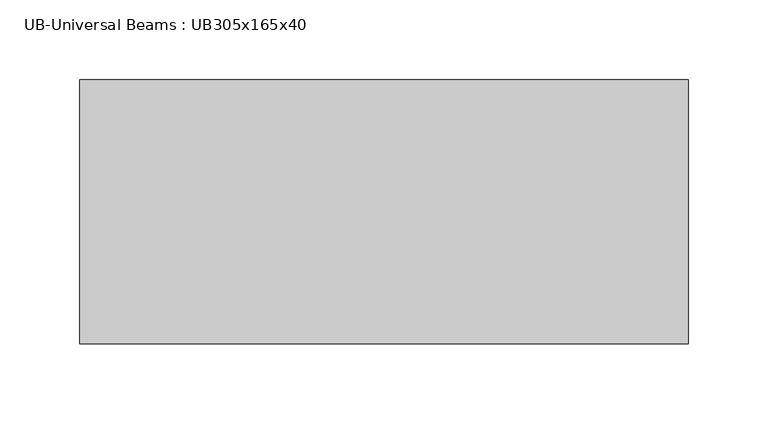
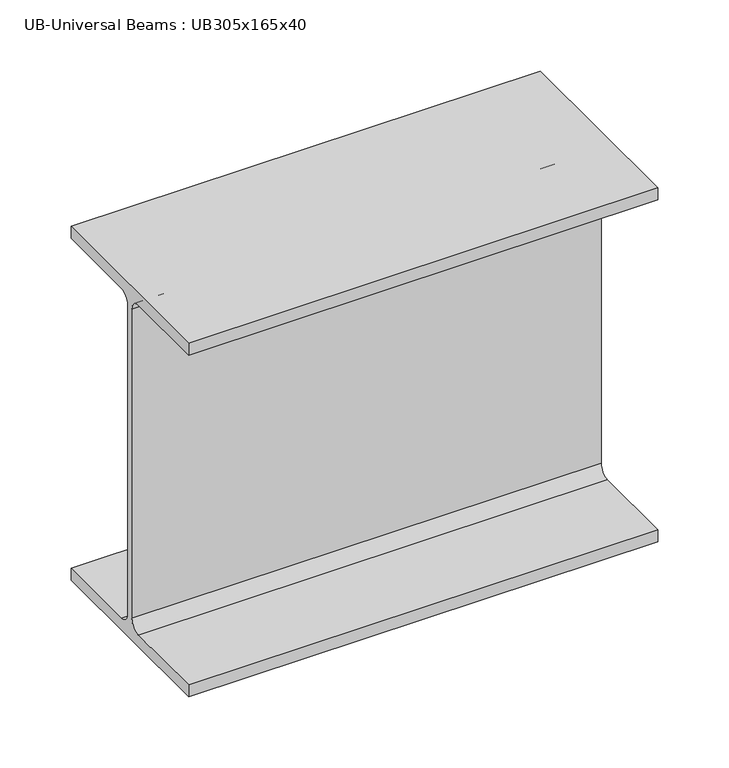
"""IFC4 building model written with IfcOpenShell, lengths in millimetres: beam geometry, UB-Universal Beams : UB305x165x40."""

from ifc_helpers import new_model, si_unit, point, frame, frame_2d, origin, place, context, project, spatial, polyline, circle_curve, trimmed, segment, composite_curve, outline, extrude, source, transform, mapped, element, save


def ub_universal_beams_ub305x165x40_928f9290(model_context):
    return source(origin(), model_context, "Body", "SweptSolid", [
        extrude(outline(composite_curve([segment(polyline([(-82.5, -141.5), (-11.9, -141.5)]), True, "CONTINUOUS"), segment(trimmed(circle_curve(frame_2d((-11.9, -132.6)), 8.9), [point((-11.9, -141.5))], [point((-3.0, -132.6))], True, "CARTESIAN"), True, "CONTINUOUS"), segment(polyline([(-3.0, -132.6), (-3.0, 132.6)]), True, "CONTINUOUS"), segment(trimmed(circle_curve(frame_2d((-11.9, 132.6)), 8.9), [point((-3.0, 132.6))], [point((-11.9, 141.5))], True, "CARTESIAN"), True, "CONTINUOUS"), segment(polyline([(-11.9, 141.5), (-82.5, 141.5), (-82.5, 151.7), (82.5, 151.7), (82.5, 141.5), (11.9, 141.5)]), True, "CONTINUOUS"), segment(trimmed(circle_curve(frame_2d((11.9, 132.6)), 8.9), [point((11.9, 141.5))], [point((3.0, 132.6))], True, "CARTESIAN"), True, "CONTINUOUS"), segment(polyline([(3.0, 132.6), (3.0, -132.6)]), True, "CONTINUOUS"), segment(trimmed(circle_curve(frame_2d((11.9, -132.6)), 8.9), [point((3.0, -132.6))], [point((11.9, -141.5))], True, "CARTESIAN"), True, "CONTINUOUS"), segment(polyline([(11.9, -141.5), (82.5, -141.5), (82.5, -151.7), (-82.5, -151.7), (-82.5, -141.5)]), True, "CONTINUOUS")], self_intersect=False)), frame((-796.35, 0.0, 0.0), z_axis=(1.0, 0.0, 0.0), x_axis=(0.0, 1.0, 0.0)), (0.0, 0.0, 1.0), 380.6),
    ])


if __name__ == "__main__":
    model = new_model("IFC4")
    model_context = context("Model", 3, world=origin())
    ifc_project = project(units=[si_unit("LENGTHUNIT", "METRE", prefix="MILLI")], contexts=[model_context])
    site = spatial("IfcSite", under=ifc_project)
    building = spatial("IfcBuilding", under=site)
    placement = place(None, origin())
    ub_universal_beams_ub305x165x40_shape = ub_universal_beams_ub305x165x40_928f9290(model_context)
    element("IfcBeam", 1, ObjectType="UB-Universal Beams : UB305x165x40", at=placement, inside=building, context=model_context, shape_type="MappedRepresentation", body=[
        mapped(ub_universal_beams_ub305x165x40_shape, transform((0.0, 0.0, 0.0), x_axis=(1.0, 0.0, 0.0), y_axis=(0.0, 1.0, 0.0), z_axis=(0.0, 0.0, 1.0))),
    ])
    save(model, "model.ifc")

# Revit data of these elements
# Type "UB-Universal Beams : UB305x165x40"
#   Section Name Key = "UB305X165X40"
#   Width = 16.5 cm
#   Web Thickness = 0.6 cm
#   Web Fillet = 0.89 cm
#   Warping Constant = 164000.0 cm⁶
#   Torsional Moment of Inertia = 14.70 cm⁴
#   Section Area = 51.3 cm²
#   Plastic Modulus weak axis = 142.0 cm³
#   Plastic Modulus strong axis = 623.0 cm³
#   Nominal Weight = 40.2999 kgf/m
#   Moment of Inertia weak axis = 764.00 cm⁴
#   Moment of Inertia strong axis = 8503.00 cm⁴
#   Height = 30.34 cm
#   Flange Thickness = 1.02 cm
#   Elastic Modulus weak axis = 92.6 cm³
#   Elastic Modulus strong axis = 560.0 cm³
#   Centroid Vertical = 15.17 cm
#   Centroid Horizontal = 8.25 cm
#   Bolt Spacing = 9.0 cm
#   Length [instance default] = 1500 mm
#   Structural Material [instance default] = Metal - Steel 43-275
#   Type Comments = ""
#   Assembly Code = ""
# Element 1 (IfcBeam, "UB-Universal Beams : UB305x165x40")
#   Materials on its faces: "Metal - Steel 43-275"
# Materials
#   "Metal - Steel 43-275": class "Metal", colour RGB 247 247 247, transparency 0, Cost = 0
